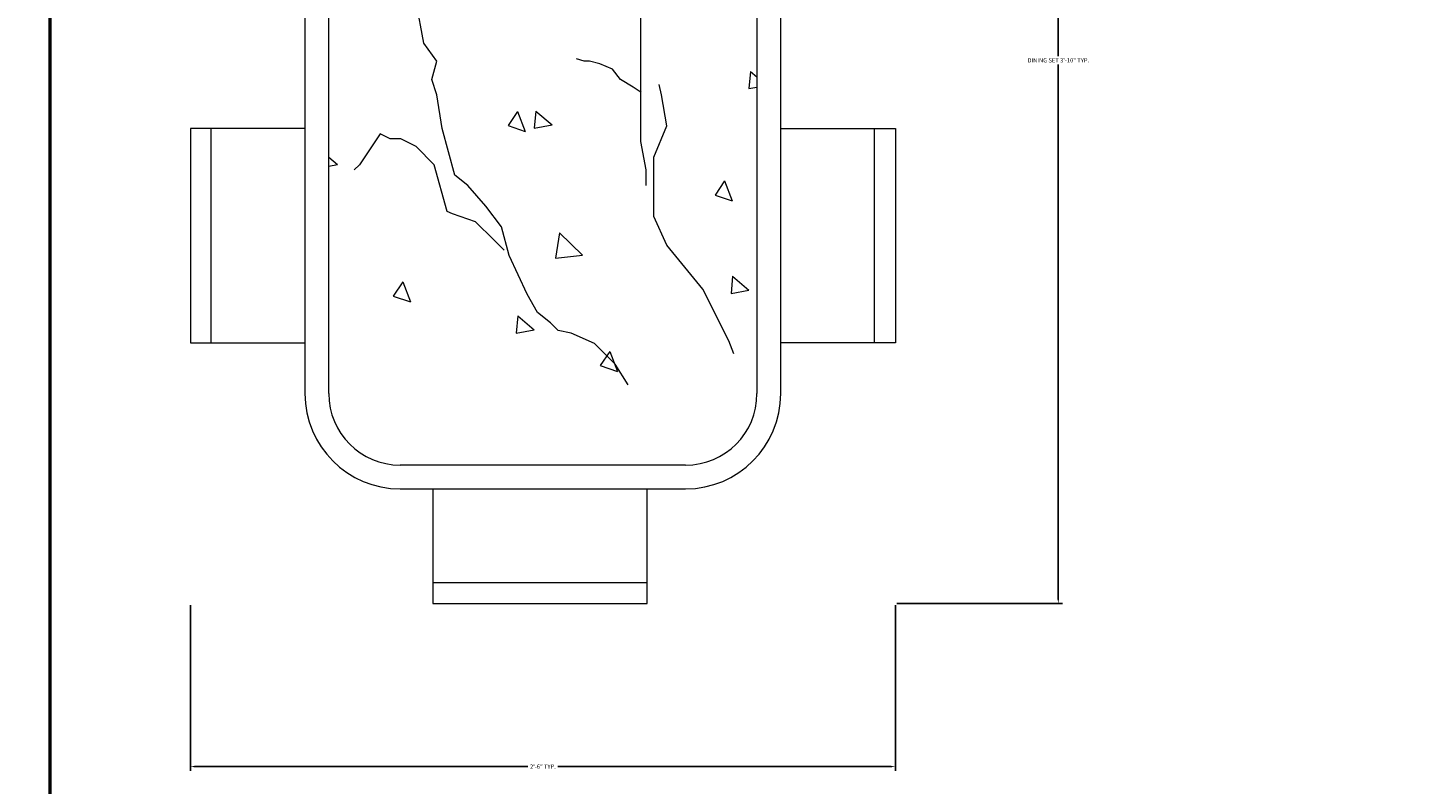
# Model space of a CAD drawing. Units: inches. Extents: x -173 to 545, y -746 to 104.
# Tile 17 of 32: x 314 to 373, y -528 to -496. Entities that reach past the tile are written whole.
import ezdxf

# ---------------------------------------------------------------- set-up
doc = ezdxf.new("R2010")
doc.units = ezdxf.units.IN
doc.header["$MEASUREMENT"] = 0
for name, color, linetype, lineweight in [('A-ANNO-DIMS', 2, 'Continuous', 18), ('A-FURN', 8, 'Continuous', 18), ('A-WALL', 7, 'Continuous', 50)]:
    doc.layers.add(name, color=color, linetype=linetype, lineweight=lineweight)
doc.styles.get("Standard").update_dxf_attribs({"font": 'arial.ttf'})
doc.dimstyles.get("Standard").update_dxf_attribs({"dimtxt": 0.18, "dimasz": 0.18, "dimexe": 0.18, "dimexo": 0.0625, "dimgap": 0.09, "dimtad": 0, "dimtih": 1, "dimtoh": 1, "dimdec": 0, "dimzin": 0, "dimdsep": 46, "dimlunit": 3, "dimtxsty": 'Standard', "dimcen": 0.09, "dimadec": 0, "dimazin": 0, "dimtfac": 1, "dimtdec": 0, "dimtofl": 0, "dimtmove": 0, "dimatfit": 3, "dimfxl": 1, "dimtolj": 1, "dimtzin": 0, "dimarcsym": 0})

# ---------------------------------------------------------------- blocks, each defined once
blk = doc.blocks.new('DINING-TABLE-SIX')
for p, q in [((4.876, 37.251), (4.876, 8.923)), ((5.888, 8.923), (5.888, 37.251)), ((24.099, 37.251), (24.099, 8.923)), ((25.11, 8.923), (25.11, 37.251)), ((19.164, 19.638), (19.164, 26.018)), ((9.934, 23.818), (9.604, 25.578)), ((10.483, 23.048), (9.934, 23.818)), ((10.264, 22.278), (10.483, 23.048)), ((16.751, 23.046), (16.421, 23.156)), ((16.97, 23.046), (16.751, 23.046)), ((17.41, 22.936), (16.97, 23.046)), ((17.959, 22.716), (17.41, 22.936)), ((18.289, 22.276), (17.959, 22.716)), ((23.82, 22.616), (23.757, 21.89)), ((23.82, 22.616), (24.099, 22.382)), ((10.483, 21.618), (10.264, 22.278)), ((18.838, 21.946), (18.289, 22.276)), ((19.168, 21.726), (18.838, 21.946)), ((20.043, 21.618), (19.933, 22.058)), ((23.756, 21.89), (24.099, 21.953)), ((10.703, 20.188), (10.483, 21.618)), ((20.263, 20.298), (20.043, 21.618)), ((13.918, 20.919), (13.511, 20.315)), ((13.918, 20.919), (14.245, 20.069)), ((14.688, 20.931), (14.625, 20.205)), ((14.688, 20.931), (15.386, 20.346)), ((4.876, 20.193), (0, 20.193)), ((0, 20.193), (0, 11.088)), ((0.89, 11.088), (0.89, 20.193)), ((8.066, 19.968), (7.187, 18.648)), ((8.505, 19.748), (8.066, 19.968)), ((11.252, 18.208), (10.703, 20.188)), ((13.511, 20.315), (14.244, 20.069)), ((14.624, 20.205), (15.385, 20.346)), ((19.713, 18.978), (20.263, 20.298)), ((25.11, 20.193), (29.987, 20.193)), ((29.097, 11.088), (29.097, 20.193)), ((29.987, 20.193), (29.987, 11.088)), ((8.945, 19.748), (8.505, 19.748)), ((9.604, 19.418), (8.945, 19.748)), ((10.373, 18.648), (9.604, 19.418)), ((19.384, 18.428), (19.164, 19.638)), ((5.888, 18.968), (6.254, 18.661)), ((19.713, 16.447), (19.713, 18.978)), ((5.888, 18.594), (6.253, 18.661)), ((7.187, 18.648), (6.967, 18.428)), ((10.923, 16.667), (10.373, 18.648)), ((11.802, 17.768), (11.252, 18.208)), ((19.384, 17.768), (19.384, 18.428)), ((12.571, 16.888), (11.802, 17.768)), ((22.722, 17.965), (22.315, 17.361)), ((22.722, 17.965), (23.048, 17.115)), ((22.314, 17.361), (23.048, 17.115)), ((11.143, 16.557), (10.923, 16.667)), ((12.132, 16.227), (11.143, 16.557)), ((13.23, 16.007), (12.571, 16.888)), ((20.263, 15.237), (19.713, 16.447)), ((12.901, 15.457), (12.132, 16.227)), ((13.56, 14.797), (13.23, 16.007)), ((13.34, 15.017), (12.901, 15.457)), ((15.694, 15.755), (15.526, 14.675)), ((15.694, 15.755), (16.679, 14.809)), ((14.329, 13.147), (13.56, 14.797)), ((15.526, 14.675), (16.679, 14.809)), ((21.801, 13.367), (20.263, 15.237)), ((9.03, 13.672), (8.623, 13.069)), ((9.03, 13.672), (9.357, 12.822)), ((23.058, 13.908), (22.995, 13.182)), ((23.058, 13.908), (23.756, 13.322)), ((8.623, 13.068), (9.356, 12.822)), ((14.769, 12.377), (14.329, 13.147)), ((22.9, 11.167), (21.801, 13.367)), ((22.994, 13.182), (23.755, 13.322)), ((15.318, 11.937), (14.769, 12.377)), ((13.926, 12.223), (13.863, 11.497)), ((13.926, 12.223), (14.624, 11.638)), ((15.648, 11.607), (15.318, 11.937)), ((13.862, 11.497), (14.623, 11.638)), ((16.197, 11.497), (15.648, 11.607)), ((17.186, 11.057), (16.197, 11.497)), ((23.12, 10.617), (22.9, 11.167)), ((0, 11.088), (4.876, 11.088)), ((18.065, 10.177), (17.186, 11.057)), ((17.834, 10.718), (17.427, 10.115)), ((17.834, 10.718), (18.16, 9.868)), ((29.987, 11.088), (25.11, 11.088)), ((17.426, 10.115), (18.16, 9.868)), ((18.615, 9.297), (18.065, 10.177)), ((21.064, 5.888), (8.923, 5.888)), ((8.923, 4.876), (21.064, 4.876)), ((10.319, 4.876), (10.319, 0)), ((19.425, 0), (19.425, 4.876)), ((19.425, 0.89), (10.319, 0.89)), ((10.319, 0), (19.425, 0))]:
    blk.add_line(p, q)
for centre, radius, start, end in [((8.923, 8.923), 4.047, 180, 270), ((8.923, 8.923), 3.035, 180, 270), ((21.064, 8.923), 3.035, 270, 0), ((21.064, 8.923), 4.047, 270, 0)]:
    blk.add_arc(centre, radius, start, end)
blk = doc.blocks.new('*D52')
at = {"layer": 'A-ANNO-DIMS', "color": 0, "lineweight": -2, "transparency": 16777216}
for p, q in [((351.326, -473.821), (358.369, -473.821)), ((358.189, -474.001), (358.189, -496.725)), ((358.189, -519.816), (358.189, -497.091)), ((351.326, -519.996), (358.369, -519.996))]:
    blk.add_line(p, q, dxfattribs=at)
at = {"layer": 'A-ANNO-DIMS', "color": 0, "transparency": 16777216}
for points in [[(358.159, -474.001), (358.219, -474.001), (358.189, -473.821)], [(358.159, -519.816), (358.219, -519.816), (358.189, -519.996)]]:
    blk.add_solid(points, dxfattribs=at)
at = {"layer": 'Defpoints', "color": 0, "transparency": 16777216}
for p in [(351.263, -473.821), (358.189, -473.821), (351.263, -519.996)]:
    blk.add_point(p, dxfattribs=at)
at = {"layer": 'A-ANNO-DIMS', "color": 0, "transparency": 16777216, "insert": (358.189, -496.908), "char_height": 0.18, "attachment_point": 5}
blk.add_mtext('\\A1;DINING SET 3\'-10" TYP.', dxfattribs=at)
blk = doc.blocks.new('*D53')
at = {"layer": 'A-ANNO-DIMS', "color": 0, "lineweight": -2, "transparency": 16777216}
for p, q in [((321.276, -520.058), (321.276, -527.102)), ((351.263, -520.058), (351.263, -527.102)), ((321.456, -526.922), (335.629, -526.922)), ((351.083, -526.922), (336.91, -526.922))]:
    blk.add_line(p, q, dxfattribs=at)
at = {"layer": 'A-ANNO-DIMS', "color": 0, "transparency": 16777216}
for points in [[(321.456, -526.892), (321.456, -526.952), (321.276, -526.922)], [(351.083, -526.892), (351.083, -526.952), (351.263, -526.922)]]:
    blk.add_solid(points, dxfattribs=at)
at = {"layer": 'Defpoints', "color": 0, "transparency": 16777216}
for p in [(321.276, -519.996), (351.263, -519.996), (351.263, -526.922)]:
    blk.add_point(p, dxfattribs=at)
at = {"layer": 'A-ANNO-DIMS', "color": 0, "transparency": 16777216, "insert": (336.27, -526.922), "char_height": 0.18, "attachment_point": 5}
blk.add_mtext('\\A1;2\'-6" TYP.', dxfattribs=at)
blk = doc.blocks.new('*D82')
at = {"layer": 'A-ANNO-DIMS', "color": 0, "lineweight": -2, "transparency": 16777216}
for p, q in [((219.864, -467.862), (545.081, -467.862)), ((544.901, -468.042), (544.901, -509.68)), ((544.901, -551.682), (544.901, -510.044)), ((219.864, -551.862), (545.081, -551.862))]:
    blk.add_line(p, q, dxfattribs=at)
at = {"layer": 'A-ANNO-DIMS', "color": 0, "transparency": 16777216}
for points in [[(544.871, -468.042), (544.931, -468.042), (544.901, -467.862)], [(544.871, -551.682), (544.931, -551.682), (544.901, -551.862)]]:
    blk.add_solid(points, dxfattribs=at)
at = {"layer": 'Defpoints', "color": 0, "transparency": 16777216}
for p in [(219.801, -467.862), (219.801, -551.862), (544.901, -551.862)]:
    blk.add_point(p, dxfattribs=at)
at = {"layer": 'A-ANNO-DIMS', "color": 0, "transparency": 16777216, "insert": (544.901, -509.862), "char_height": 0.18, "attachment_point": 5}
blk.add_mtext('\\A1;7\'-0"', dxfattribs=at)

msp = doc.modelspace()

# ---------------------------------------------------------------- linework, layer by layer
at = {"layer": 'A-WALL'}
msp.add_line((315.301, -463.362), (315.301, -560.862), dxfattribs=at)

# ---------------------------------------------------------------- block references
at = {"layer": 'A-FURN'}
msp.add_blockref('DINING-TABLE-SIX', (321.276, -519.995), dxfattribs=at)

# ---------------------------------------------------------------- dimensions: what is measured, and where the dimension line sits
at = {"layer": 'A-ANNO-DIMS'}
dim = msp.add_linear_dim(base=(544.901, -551.862), p1=(219.801, -467.862), p2=(219.801, -551.862), angle=90, dimstyle='Standard', override={"dimdec": 1, "dimlfac": 1, "dimrnd": 0, "dimzin": 1, "dimdsep": 46, "dimlunit": 4, "dimfrac": 2}, dxfattribs=at)
dim.commit()
dim.dimension.update_dxf_attribs({"geometry": '*D82', "text_midpoint": (544.901, -509.862)})
dim = msp.add_linear_dim(base=(358.189, -473.821), p1=(351.263, -519.996), p2=(351.263, -473.821), angle=90, text='DINING SET <> TYP.', dimstyle='Standard', override={"dimdec": 1, "dimlfac": 1, "dimrnd": 0, "dimzin": 1, "dimdsep": 46, "dimlunit": 4, "dimfrac": 2}, dxfattribs=at)
dim.commit()
dim.dimension.update_dxf_attribs({"geometry": '*D52', "text_midpoint": (358.189, -496.908)})
dim = msp.add_linear_dim(base=(351.263, -526.922), p1=(321.276, -519.996), p2=(351.263, -519.996), text='<> TYP.', dimstyle='Standard', override={"dimdec": 1, "dimlfac": 1, "dimrnd": 0, "dimzin": 1, "dimdsep": 46, "dimlunit": 4, "dimfrac": 2}, dxfattribs=at)
dim.commit()
dim.dimension.update_dxf_attribs({"geometry": '*D53', "text_midpoint": (336.27, -526.922)})

doc.saveas('drawing.dxf')
